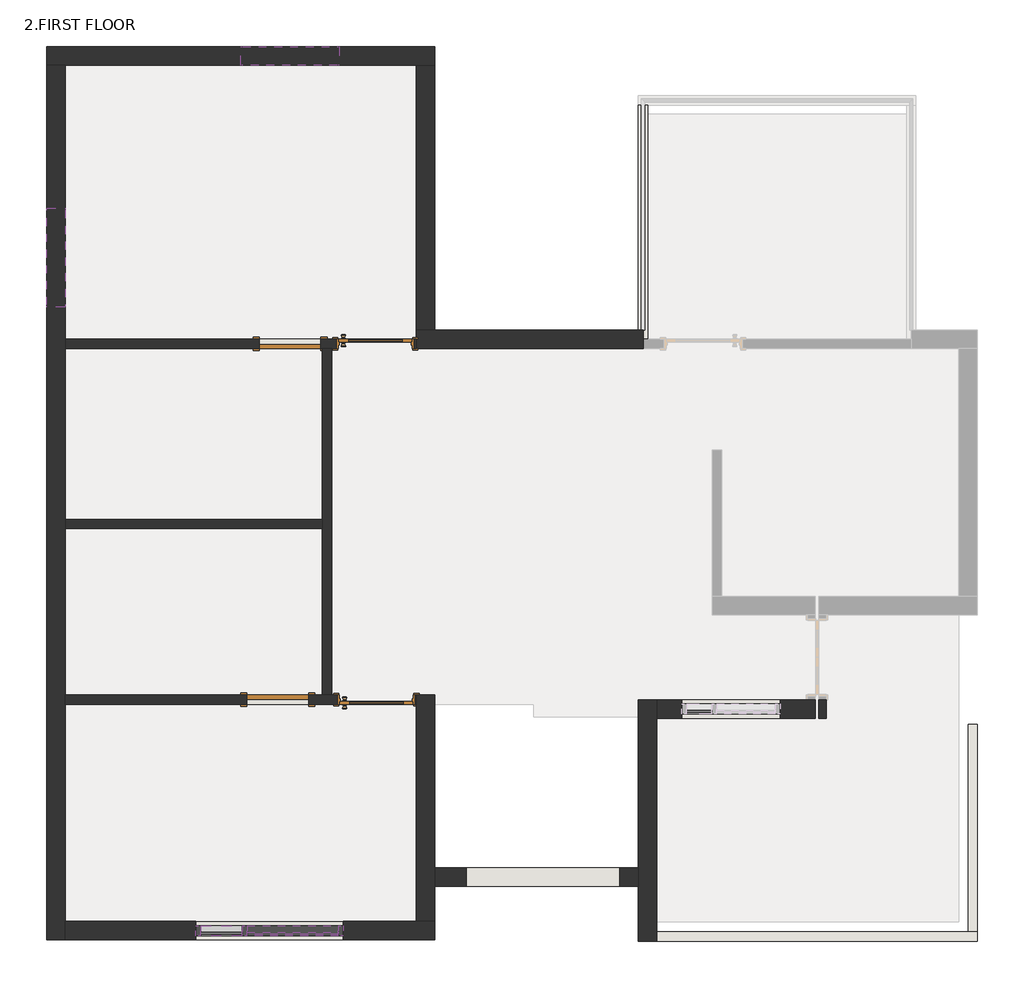
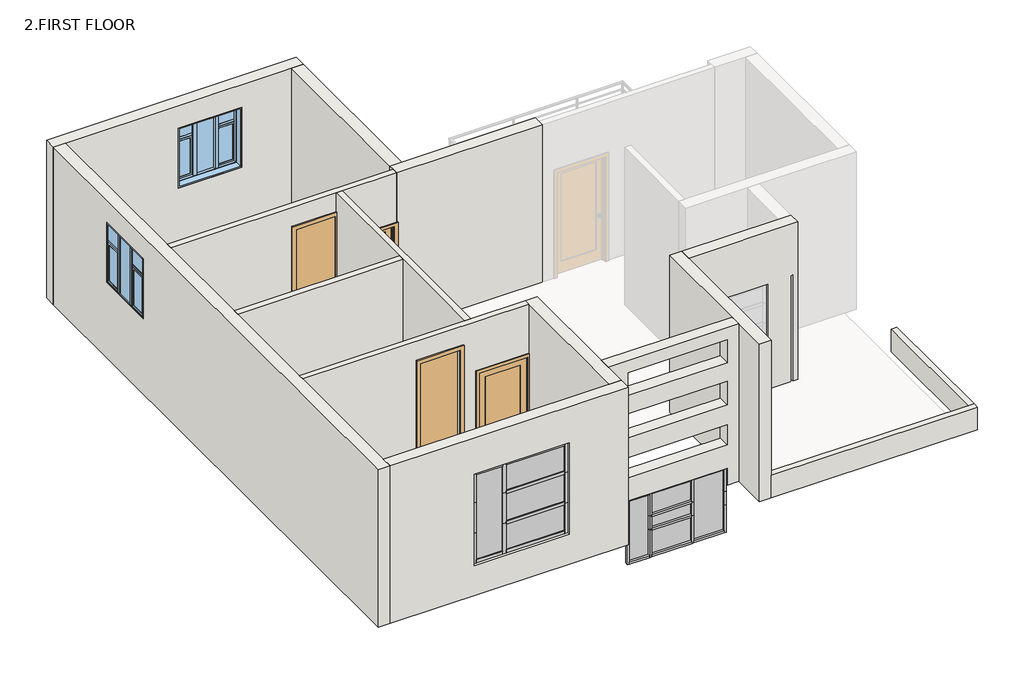
# One storey, part 1 of 2: 35 members, 16 walls, 10 plates, 4 doors, 2 windows.
"""IFC4 building model written with IfcOpenShell, lengths in millimetres."""

from ifc_helpers import new_model, si_unit, frame, origin, place, context, project, spatial, polyline, outline, extrude, faceted_brep, transform, mapped, element, save
from components import door_interior_single_1_panel_wood_4_x7_a3feeac7, door_interior_single_1_panel_wood_4_x7_3c6ab76a, door_214872d5, door_78caadf7, member_ade56e03, member_acd33549, member_5e1cd3ea, member_0748a5fc, member_494741c6, member_55e892ad, member_6a2c51b8, member_01c630bb, member_9157fb7c, member_e8de63ac, member_0b7646a3, member_e6b9f524, member_2cd1b1d9, member_866a01fa, member_c3a59c23, system_panel_glazed_06acdacc, system_panel_glazed_f6e37d5f, system_panel_glazed_d1e8daba, system_panel_glazed_58042333, system_panel_glazed_55b634e8, system_panel_glazed_1f22f3a7, system_panel_glazed_63219d49, system_panel_glazed_1b2af392, system_panel_glazed_fe088b68, window_casement_triple_side_transom_4_x4_fd24aed3

model = new_model("IFC4")

# Units and contexts
model_context = context("Model", 3, world=origin())
ifc_project = project(units=[si_unit("LENGTHUNIT", "METRE", prefix="MILLI")], contexts=[model_context])

# Site, building, storey
site = spatial("IfcSite", under=ifc_project)
building = spatial("IfcBuilding", under=site)
storey = spatial("IfcBuildingStorey", under=building, Name="2.FIRST FLOOR", Elevation=3810.0)

# Doors
placement = place(None, origin())
door_interior_single_1_panel_wood_4_x7_shape = door_interior_single_1_panel_wood_4_x7_a3feeac7(model_context)
element("IfcDoor", 1, ObjectType="Door-Interior-Single-1_Panel-Wood : 4'X7'", at=placement, inside=storey, context=model_context, shape_type="MappedRepresentation", body=[
    mapped(door_interior_single_1_panel_wood_4_x7_shape, transform((-3488.3749552, 2247.2410289, 3810.0), x_axis=(1.0, 0.0, 0.0), y_axis=(0.0, 1.0, 0.0), z_axis=(0.0, 0.0, 1.0))),
])
door_interior_single_1_panel_wood_4_x7_2_shape = door_interior_single_1_panel_wood_4_x7_3c6ab76a(model_context)
element("IfcDoor", 2, ObjectType="Door-Interior-Single-1_Panel-Wood : 4'X7'", at=placement, inside=storey, context=model_context, shape_type="MappedRepresentation", body=[
    mapped(door_interior_single_1_panel_wood_4_x7_2_shape, transform((-3501.0749552, 6654.1410289, 3810.0), x_axis=(1.0, 0.0, 0.0), y_axis=(0.0, 1.0, 0.0), z_axis=(0.0, 0.0, 1.0))),
])
door_shape = door_214872d5(model_context)
element("IfcDoor", 3, ObjectType="Single-Flush : 2'6\" X 7'", at=placement, inside=storey, context=model_context, shape_type="MappedRepresentation", body=[
    mapped(door_shape, transform((-4707.5749552, 2250.4160289, 4419.6), x_axis=(1.0, 0.0, 0.0), y_axis=(0.0, 1.0, 0.0), z_axis=(0.0, 0.0, 1.0))),
])
door_2_shape = door_78caadf7(model_context)
element("IfcDoor", 4, ObjectType="Single-Flush : 2'6\" X 7'", at=placement, inside=storey, context=model_context, shape_type="MappedRepresentation", body=[
    mapped(door_2_shape, transform((-4555.1749552, 6650.9660289, 4419.6), x_axis=(1.0, 0.0, 0.0), y_axis=(0.0, 1.0, 0.0), z_axis=(0.0, 0.0, 1.0))),
])

# Members
member_shape = member_ade56e03(model_context)
element("IfcMember", 5, ObjectType="Rectangular Mullion : 1.5\" x 2.5\" rectangular", at=placement, inside=storey, context=model_context, shape_type="MappedRepresentation", body=[
    mapped(member_shape, transform((-2380.0564961, 2.5160289, 4161.1588836), x_axis=(-1.0, 0.0, 0.0), y_axis=(0.0, -1.0, 0.0), z_axis=(0.0, 0.0, 1.0))),
])
element("IfcMember", 6, ObjectType="Rectangular Mullion : 1.5\" x 2.5\" rectangular", at=placement, inside=storey, context=model_context, shape_type="MappedRepresentation", body=[
    mapped(member_shape, transform((-478.4749552, 2.5160289, 3680.9734267), x_axis=(1.0, 0.0, 0.0), y_axis=(0.0, -1.0, 0.0), z_axis=(0.0, 0.0, -1.0))),
])
member_2_shape = member_acd33549(model_context)
element("IfcMember", 7, ObjectType="Rectangular Mullion : 1.5\" x 2.5\" rectangular", at=placement, inside=storey, context=model_context, shape_type="MappedRepresentation", body=[
    mapped(member_2_shape, transform((-478.4749552, 2.5160289, 2845.1879698), x_axis=(1.0, 0.0, 0.0), y_axis=(0.0, -1.0, 0.0), z_axis=(0.0, 0.0, -1.0))),
])
member_3_shape = member_5e1cd3ea(model_context)
element("IfcMember", 8, ObjectType="Rectangular Mullion : 1.5\" x 2.5\" rectangular", at=placement, inside=storey, context=model_context, shape_type="MappedRepresentation", body=[
    mapped(member_3_shape, transform((-2380.0564961, 2.5160289, 3680.9734267), x_axis=(-1.0, 0.0, 0.0), y_axis=(0.0, -1.0, 0.0), z_axis=(0.0, 0.0, 1.0))),
])
element("IfcMember", 9, ObjectType="Rectangular Mullion : 1.5\" x 2.5\" rectangular", at=placement, inside=storey, context=model_context, shape_type="MappedRepresentation", body=[
    mapped(member_3_shape, transform((-478.4749552, 2.5160289, 3402.3782744), x_axis=(1.0, 0.0, 0.0), y_axis=(0.0, -1.0, 0.0), z_axis=(0.0, 0.0, -1.0))),
])
element("IfcMember", 10, ObjectType="Rectangular Mullion : 1.5\" x 2.5\" rectangular", at=placement, inside=storey, context=model_context, shape_type="MappedRepresentation", body=[
    mapped(member_2_shape, transform((-2380.0564961, 2.5160289, 3402.3782744), x_axis=(-1.0, 0.0, 0.0), y_axis=(0.0, -1.0, 0.0), z_axis=(0.0, 0.0, 1.0))),
])
member_4_shape = member_0748a5fc(model_context)
element("IfcMember", 11, ObjectType="Rectangular Mullion : 1.5\" x 2.5\" rectangular", at=placement, inside=storey, context=model_context, shape_type="MappedRepresentation", body=[
    mapped(member_4_shape, transform((-1913.5749552, 2.5160289, 2845.1879698), x_axis=(0.0, 0.0, -1.0), y_axis=(0.0, -1.0, 0.0), z_axis=(-1.0, 0.0, 0.0))),
])
element("IfcMember", 12, ObjectType="Rectangular Mullion : 1.5\" x 2.5\" rectangular", at=placement, inside=storey, context=model_context, shape_type="MappedRepresentation", body=[
    mapped(member_4_shape, transform((-1138.8749552, 2.5160289, 4161.1588836), x_axis=(0.0, 0.0, 1.0), y_axis=(0.0, -1.0, 0.0), z_axis=(1.0, 0.0, 0.0))),
])
member_5_shape = member_494741c6(model_context)
element("IfcMember", 13, ObjectType="Rectangular Mullion : 1.5\" x 2.5\" rectangular", at=placement, inside=storey, context=model_context, shape_type="MappedRepresentation", body=[
    mapped(member_5_shape, transform((-1932.6249552, 2.5160289, 2845.1879698), x_axis=(1.0, 0.0, 0.0), y_axis=(0.0, -1.0, 0.0), z_axis=(0.0, 0.0, -1.0))),
])
element("IfcMember", 14, ObjectType="Rectangular Mullion : 1.5\" x 2.5\" rectangular", at=placement, inside=storey, context=model_context, shape_type="MappedRepresentation", body=[
    mapped(member_5_shape, transform((-1119.8249552, 2.5160289, 2845.1879698), x_axis=(1.0, 0.0, 0.0), y_axis=(0.0, -1.0, 0.0), z_axis=(0.0, 0.0, -1.0))),
])
member_6_shape = member_55e892ad(model_context)
element("IfcMember", 15, ObjectType="Rectangular Mullion : 1.5\" x 2.5\" rectangular", at=placement, inside=storey, context=model_context, shape_type="MappedRepresentation", body=[
    mapped(member_6_shape, transform((-1138.8749552, 2.5160289, 3680.9734267), x_axis=(0.0, 0.0, 1.0), y_axis=(0.0, -1.0, 0.0), z_axis=(1.0, 0.0, 0.0))),
])
element("IfcMember", 16, ObjectType="Rectangular Mullion : 1.5\" x 2.5\" rectangular", at=placement, inside=storey, context=model_context, shape_type="MappedRepresentation", body=[
    mapped(member_6_shape, transform((-1138.8749552, 2.5160289, 3402.3782744), x_axis=(0.0, 0.0, 1.0), y_axis=(0.0, -1.0, 0.0), z_axis=(1.0, 0.0, 0.0))),
])
member_7_shape = member_6a2c51b8(model_context)
element("IfcMember", 17, ObjectType="Rectangular Mullion : 1.5\" x 2.5\" rectangular", at=placement, inside=storey, context=model_context, shape_type="MappedRepresentation", body=[
    mapped(member_7_shape, transform((-1932.6249552, 2.5160289, 3680.9734267), x_axis=(1.0, 0.0, 0.0), y_axis=(0.0, -1.0, 0.0), z_axis=(0.0, 0.0, -1.0))),
])
element("IfcMember", 18, ObjectType="Rectangular Mullion : 1.5\" x 2.5\" rectangular", at=placement, inside=storey, context=model_context, shape_type="MappedRepresentation", body=[
    mapped(member_7_shape, transform((-1119.8249552, 2.5160289, 3680.9734267), x_axis=(1.0, 0.0, 0.0), y_axis=(0.0, -1.0, 0.0), z_axis=(0.0, 0.0, -1.0))),
])
member_8_shape = member_01c630bb(model_context)
element("IfcMember", 19, ObjectType="Rectangular Mullion : 1.5\" x 2.5\" rectangular", at=placement, inside=storey, context=model_context, shape_type="MappedRepresentation", body=[
    mapped(member_8_shape, transform((-1932.6249552, 2.5160289, 3402.3782744), x_axis=(1.0, 0.0, 0.0), y_axis=(0.0, -1.0, 0.0), z_axis=(0.0, 0.0, -1.0))),
])
element("IfcMember", 20, ObjectType="Rectangular Mullion : 1.5\" x 2.5\" rectangular", at=placement, inside=storey, context=model_context, shape_type="MappedRepresentation", body=[
    mapped(member_8_shape, transform((-1119.8249552, 2.5160289, 3402.3782744), x_axis=(1.0, 0.0, 0.0), y_axis=(0.0, -1.0, 0.0), z_axis=(0.0, 0.0, -1.0))),
])
member_9_shape = member_9157fb7c(model_context)
element("IfcMember", 21, ObjectType="Rectangular Mullion : 1.5\" x 2.5\" rectangular", at=placement, inside=storey, context=model_context, shape_type="MappedRepresentation", body=[
    mapped(member_9_shape, transform((-2341.9564961, 2.5160289, 2845.1879698), x_axis=(0.0, 0.0, -1.0), y_axis=(0.0, -1.0, 0.0), z_axis=(-1.0, 0.0, 0.0))),
])
element("IfcMember", 22, ObjectType="Rectangular Mullion : 1.5\" x 2.5\" rectangular", at=placement, inside=storey, context=model_context, shape_type="MappedRepresentation", body=[
    mapped(member_9_shape, transform((-1951.6749552, 2.5160289, 4161.1588836), x_axis=(0.0, 0.0, 1.0), y_axis=(0.0, -1.0, 0.0), z_axis=(1.0, 0.0, 0.0))),
])
member_10_shape = member_e8de63ac(model_context)
element("IfcMember", 23, ObjectType="Rectangular Mullion : 1.5\" x 2.5\" rectangular", at=placement, inside=storey, context=model_context, shape_type="MappedRepresentation", body=[
    mapped(member_10_shape, transform((-516.5749552, 2.5160289, 4161.1588836), x_axis=(0.0, 0.0, 1.0), y_axis=(0.0, -1.0, 0.0), z_axis=(1.0, 0.0, 0.0))),
])
element("IfcMember", 24, ObjectType="Rectangular Mullion : 1.5\" x 2.5\" rectangular", at=placement, inside=storey, context=model_context, shape_type="MappedRepresentation", body=[
    mapped(member_10_shape, transform((-1100.7749552, 2.5160289, 2845.1879698), x_axis=(0.0, 0.0, -1.0), y_axis=(0.0, -1.0, 0.0), z_axis=(-1.0, 0.0, 0.0))),
])
member_11_shape = member_0b7646a3(model_context)
element("IfcMember", 25, ObjectType="Rectangular Mullion : 2.5\" x 5\" rectangular", at=placement, inside=storey, context=model_context, shape_type="MappedRepresentation", body=[
    mapped(member_11_shape, transform((-5660.0749552, -607.0839711, 6273.8), x_axis=(0.0, 0.0, 1.0), y_axis=(0.0, 1.0, 0.0), z_axis=(-1.0, 0.0, 0.0))),
])
member_12_shape = member_e6b9f524(model_context)
element("IfcMember", 26, ObjectType="Rectangular Mullion : 2.5\" x 5\" rectangular", at=placement, inside=storey, context=model_context, shape_type="MappedRepresentation", body=[
    mapped(member_12_shape, transform((-3958.2749552, -607.0839711, 4419.6), x_axis=(0.0, 0.0, -1.0), y_axis=(0.0, 1.0, 0.0), z_axis=(1.0, 0.0, 0.0))),
])
member_13_shape = member_2cd1b1d9(model_context)
element("IfcMember", 27, ObjectType="Rectangular Mullion : 2.5\" x 5\" rectangular", at=placement, inside=storey, context=model_context, shape_type="MappedRepresentation", body=[
    mapped(member_13_shape, transform((-5113.9749552, -607.0839711, 4419.6), x_axis=(-1.0, 0.0, 0.0), y_axis=(0.0, 1.0, 0.0), z_axis=(0.0, 0.0, -1.0))),
])
member_14_shape = member_866a01fa(model_context)
element("IfcMember", 28, ObjectType="Rectangular Mullion : 2.5\" x 5\" rectangular", at=placement, inside=storey, context=model_context, shape_type="MappedRepresentation", body=[
    mapped(member_14_shape, transform((-5082.2249552, -607.0839711, 5655.7333333), x_axis=(0.0, 0.0, 1.0), y_axis=(0.0, 1.0, 0.0), z_axis=(-1.0, 0.0, 0.0))),
])
element("IfcMember", 29, ObjectType="Rectangular Mullion : 2.5\" x 5\" rectangular", at=placement, inside=storey, context=model_context, shape_type="MappedRepresentation", body=[
    mapped(member_14_shape, transform((-5082.2249552, -607.0839711, 5037.6666667), x_axis=(0.0, 0.0, 1.0), y_axis=(0.0, 1.0, 0.0), z_axis=(-1.0, 0.0, 0.0))),
])
element("IfcMember", 30, ObjectType="Rectangular Mullion : 2.5\" x 5\" rectangular", at=placement, inside=storey, context=model_context, shape_type="MappedRepresentation", body=[
    mapped(member_11_shape, transform((-5145.7249552, -607.0839711, 4419.6), x_axis=(0.0, 0.0, -1.0), y_axis=(0.0, 1.0, 0.0), z_axis=(1.0, 0.0, 0.0))),
])
element("IfcMember", 31, ObjectType="Rectangular Mullion : 2.5\" x 5\" rectangular", at=placement, inside=storey, context=model_context, shape_type="MappedRepresentation", body=[
    mapped(member_12_shape, transform((-5082.2249552, -607.0839711, 6273.8), x_axis=(0.0, 0.0, 1.0), y_axis=(0.0, 1.0, 0.0), z_axis=(-1.0, 0.0, 0.0))),
])
element("IfcMember", 32, ObjectType="Rectangular Mullion : 2.5\" x 5\" rectangular", at=placement, inside=storey, context=model_context, shape_type="MappedRepresentation", body=[
    mapped(member_13_shape, transform((-5113.9749552, -607.0839711, 5655.7333333), x_axis=(-1.0, 0.0, 0.0), y_axis=(0.0, 1.0, 0.0), z_axis=(0.0, 0.0, -1.0))),
])
element("IfcMember", 33, ObjectType="Rectangular Mullion : 2.5\" x 5\" rectangular", at=placement, inside=storey, context=model_context, shape_type="MappedRepresentation", body=[
    mapped(member_13_shape, transform((-5113.9749552, -607.0839711, 5037.6666667), x_axis=(-1.0, 0.0, 0.0), y_axis=(0.0, 1.0, 0.0), z_axis=(0.0, 0.0, -1.0))),
])
member_15_shape = member_c3a59c23(model_context)
element("IfcMember", 34, ObjectType="Rectangular Mullion : 2.5\" x 5\" rectangular", at=placement, inside=storey, context=model_context, shape_type="MappedRepresentation", body=[
    mapped(member_15_shape, transform((-3894.7749552, -607.0839711, 6273.8), x_axis=(1.0, 0.0, 0.0), y_axis=(0.0, 1.0, 0.0), z_axis=(0.0, 0.0, 1.0))),
])
element("IfcMember", 35, ObjectType="Rectangular Mullion : 2.5\" x 5\" rectangular", at=placement, inside=storey, context=model_context, shape_type="MappedRepresentation", body=[
    mapped(member_15_shape, transform((-5723.5749552, -607.0839711, 4419.6), x_axis=(-1.0, 0.0, 0.0), y_axis=(0.0, 1.0, 0.0), z_axis=(0.0, 0.0, -1.0))),
])
element("IfcMember", 36, ObjectType="Rectangular Mullion : 2.5\" x 5\" rectangular", at=placement, inside=storey, context=model_context, shape_type="MappedRepresentation", body=[
    mapped(member_15_shape, transform((-5723.5749552, -607.0839711, 5655.7333333), x_axis=(-1.0, 0.0, 0.0), y_axis=(0.0, 1.0, 0.0), z_axis=(0.0, 0.0, -1.0))),
])
element("IfcMember", 37, ObjectType="Rectangular Mullion : 2.5\" x 5\" rectangular", at=placement, inside=storey, context=model_context, shape_type="MappedRepresentation", body=[
    mapped(member_15_shape, transform((-5723.5749552, -607.0839711, 5037.6666667), x_axis=(-1.0, 0.0, 0.0), y_axis=(0.0, 1.0, 0.0), z_axis=(0.0, 0.0, -1.0))),
])
element("IfcMember", 38, ObjectType="Rectangular Mullion : 2.5\" x 5\" rectangular", at=placement, inside=storey, context=model_context, shape_type="MappedRepresentation", body=[
    mapped(member_15_shape, transform((-3894.7749552, -607.0839711, 5655.7333333), x_axis=(1.0, 0.0, 0.0), y_axis=(0.0, 1.0, 0.0), z_axis=(0.0, 0.0, 1.0))),
])
element("IfcMember", 39, ObjectType="Rectangular Mullion : 2.5\" x 5\" rectangular", at=placement, inside=storey, context=model_context, shape_type="MappedRepresentation", body=[
    mapped(member_15_shape, transform((-3894.7749552, -607.0839711, 5037.6666667), x_axis=(1.0, 0.0, 0.0), y_axis=(0.0, 1.0, 0.0), z_axis=(0.0, 0.0, 1.0))),
])

# Plates
system_panel_glazed_shape = system_panel_glazed_06acdacc(model_context)
element("IfcPlate", 40, ObjectType="System Panel : Glazed", at=placement, inside=storey, context=model_context, shape_type="MappedRepresentation", body=[
    mapped(system_panel_glazed_shape, transform((-4520.2499552, -607.0839711, 4483.1), x_axis=(-1.0, 0.0, 0.0), y_axis=(0.0, -1.0, 0.0), z_axis=(0.0, 0.0, 1.0))),
])
element("IfcPlate", 41, ObjectType="System Panel : Glazed", at=placement, inside=storey, context=model_context, shape_type="MappedRepresentation", body=[
    mapped(system_panel_glazed_shape, transform((-4520.2499552, -607.0839711, 5687.4833333), x_axis=(-1.0, 0.0, 0.0), y_axis=(0.0, -1.0, 0.0), z_axis=(0.0, 0.0, 1.0))),
])
system_panel_glazed_2_shape = system_panel_glazed_f6e37d5f(model_context)
element("IfcPlate", 42, ObjectType="System Panel : Glazed", at=placement, inside=storey, context=model_context, shape_type="MappedRepresentation", body=[
    mapped(system_panel_glazed_2_shape, transform((-5402.8999552, -607.0839711, 4483.1), x_axis=(-1.0, 0.0, 0.0), y_axis=(0.0, -1.0, 0.0), z_axis=(0.0, 0.0, 1.0))),
])
system_panel_glazed_3_shape = system_panel_glazed_d1e8daba(model_context)
element("IfcPlate", 43, ObjectType="System Panel : Glazed", at=placement, inside=storey, context=model_context, shape_type="MappedRepresentation", body=[
    mapped(system_panel_glazed_3_shape, transform((-4520.2499552, -607.0839711, 5069.4166667), x_axis=(-1.0, 0.0, 0.0), y_axis=(0.0, -1.0, 0.0), z_axis=(0.0, 0.0, 1.0))),
])
system_panel_glazed_4_shape = system_panel_glazed_58042333(model_context)
element("IfcPlate", 44, ObjectType="System Panel : Glazed", at=placement, inside=storey, context=model_context, shape_type="MappedRepresentation", body=[
    mapped(system_panel_glazed_4_shape, transform((502.6000448, 2136.1160289, 4787.9), x_axis=(-1.0, 0.0, 0.0), y_axis=(0.0, -1.0, 0.0), z_axis=(0.0, 0.0, 1.0))),
])
system_panel_glazed_5_shape = system_panel_glazed_55b634e8(model_context)
element("IfcPlate", 45, ObjectType="System Panel : Glazed", at=placement, inside=storey, context=model_context, shape_type="MappedRepresentation", body=[
    mapped(system_panel_glazed_5_shape, transform((-1526.2249552, 2.5160289, 2883.2879698), x_axis=(1.0, 0.0, 0.0), y_axis=(0.0, 1.0, 0.0), z_axis=(0.0, 0.0, 1.0))),
])
system_panel_glazed_6_shape = system_panel_glazed_1f22f3a7(model_context)
element("IfcPlate", 46, ObjectType="System Panel : Glazed", at=placement, inside=storey, context=model_context, shape_type="MappedRepresentation", body=[
    mapped(system_panel_glazed_6_shape, transform((-1526.2249552, 2.5160289, 3700.0234267), x_axis=(1.0, 0.0, 0.0), y_axis=(0.0, 1.0, 0.0), z_axis=(0.0, 0.0, 1.0))),
])
system_panel_glazed_7_shape = system_panel_glazed_63219d49(model_context)
element("IfcPlate", 47, ObjectType="System Panel : Glazed", at=placement, inside=storey, context=model_context, shape_type="MappedRepresentation", body=[
    mapped(system_panel_glazed_7_shape, transform((-1526.2249552, 2.5160289, 3421.4282744), x_axis=(1.0, 0.0, 0.0), y_axis=(0.0, 1.0, 0.0), z_axis=(0.0, 0.0, 1.0))),
])
system_panel_glazed_8_shape = system_panel_glazed_1b2af392(model_context)
element("IfcPlate", 48, ObjectType="System Panel : Glazed", at=placement, inside=storey, context=model_context, shape_type="MappedRepresentation", body=[
    mapped(system_panel_glazed_8_shape, transform((-2146.8157257, 2.5160289, 2883.2879698), x_axis=(1.0, 0.0, 0.0), y_axis=(0.0, 1.0, 0.0), z_axis=(0.0, 0.0, 1.0))),
])
system_panel_glazed_9_shape = system_panel_glazed_fe088b68(model_context)
element("IfcPlate", 49, ObjectType="System Panel : Glazed", at=placement, inside=storey, context=model_context, shape_type="MappedRepresentation", body=[
    mapped(system_panel_glazed_9_shape, transform((-808.6749552, 2.5160289, 2883.2879698), x_axis=(1.0, 0.0, 0.0), y_axis=(0.0, 1.0, 0.0), z_axis=(0.0, 0.0, 1.0))),
])

# Walls
element("IfcWall", 50, ObjectType="4.5\" wall", at=placement, inside=storey, context=model_context, shape_type="Brep", body=[
    faceted_brep([(-7336.4749552, 6708.1160289, 7010.4), (-2993.0749552, 6708.1160289, 7010.4), (-2993.0749552, 6708.1160289, 3810.0), (-3018.4749552, 6708.1160289, 3810.0), (-3018.4749552, 6708.1160289, 5969.0), (-3983.6749552, 6708.1160289, 5969.0), (-3983.6749552, 6708.1160289, 3810.0), (-7336.4749552, 6708.1160289, 3810.0), (-4936.1749552, 6708.1160289, 4419.6), (-4174.1749552, 6708.1160289, 4419.6), (-4174.1749552, 6708.1160289, 6553.2), (-4936.1749552, 6708.1160289, 6553.2), (-2993.0749552, 6593.8160289, 7010.4), (-4040.8249552, 6593.8160289, 7010.4), (-4155.1249552, 6593.8160289, 7010.4), (-7336.4749552, 6593.8160289, 7010.4), (-7336.4749552, 6593.8160289, 3810.0), (-4155.1249552, 6593.8160289, 3810.0), (-4040.8249552, 6593.8160289, 3810.0), (-3983.6749552, 6593.8160289, 3810.0), (-3983.6749552, 6593.8160289, 5969.0), (-3018.4749552, 6593.8160289, 5969.0), (-3018.4749552, 6593.8160289, 3810.0), (-2993.0749552, 6593.8160289, 3810.0), (-4174.1749552, 6593.8160289, 4419.6), (-4936.1749552, 6593.8160289, 4419.6), (-4936.1749552, 6593.8160289, 6553.2), (-4174.1749552, 6593.8160289, 6553.2)], [[[0, 1, 2, 3, 4, 5, 6, 7], [8, 9, 10, 11]], [[12, 13, 14, 15, 16, 17, 18, 19, 20, 21, 22, 23], [24, 25, 26, 27]], [[2, 23, 22, 3]], [[16, 7, 6, 19, 18, 17]], [[1, 0, 15, 14, 13, 12]], [[21, 4, 3, 22]], [[4, 21, 20, 5]], [[5, 20, 19, 6]], [[9, 8, 25, 24]], [[10, 9, 24, 27]], [[11, 10, 27, 26]], [[8, 11, 26, 25]], [[2, 1, 12, 23]], [[0, 7, 16, 15]]]),
])
element("IfcWall", 51, ObjectType="4.5\" wall", at=placement, inside=storey, context=model_context, shape_type="Brep", body=[
    faceted_brep([(-4155.1249552, 6593.8160289, 3810.0), (-4155.1249552, 4479.2660289, 3810.0), (-4155.1249552, 4364.9660289, 3810.0), (-4155.1249552, 2307.5660289, 3810.0), (-4155.1249552, 2307.5660289, 7010.4), (-4155.1249552, 4364.9660289, 7010.4), (-4155.1249552, 4479.2660289, 7010.4), (-4155.1249552, 6593.8160289, 7010.4), (-4040.8249552, 6593.8160289, 3810.0), (-4040.8249552, 6593.8160289, 7010.4), (-4040.8249552, 2307.5660289, 7010.4), (-4040.8249552, 2307.5660289, 3810.0)], [[[0, 1, 2, 3, 4, 5, 6, 7]], [[8, 9, 10, 11]], [[3, 2, 1, 0, 8, 11]], [[7, 6, 5, 4, 10, 9]], [[0, 7, 9, 8]], [[4, 3, 11, 10]]]),
])
element("IfcWall", 52, ObjectType="4.5\" wall", at=placement, inside=storey, context=model_context, shape_type="Brep", body=[
    faceted_brep([(-7336.4749552, 2307.5660289, 7010.4), (-4155.1249552, 2307.5660289, 7010.4), (-4040.8249552, 2307.5660289, 7010.4), (-2993.0749552, 2307.5660289, 7010.4), (-2993.0749552, 2307.5660289, 3810.0), (-3005.7749552, 2307.5660289, 3810.0), (-3005.7749552, 2307.5660289, 5969.0), (-3970.9749552, 2307.5660289, 5969.0), (-3970.9749552, 2307.5660289, 3810.0), (-4040.8249552, 2307.5660289, 3810.0), (-4155.1249552, 2307.5660289, 3810.0), (-7336.4749552, 2307.5660289, 3810.0), (-5088.5749552, 2307.5660289, 4419.6), (-4326.5749552, 2307.5660289, 4419.6), (-4326.5749552, 2307.5660289, 6553.2), (-5088.5749552, 2307.5660289, 6553.2), (-2993.0749552, 2193.2660289, 7010.4), (-7336.4749552, 2193.2660289, 7010.4), (-7336.4749552, 2193.2660289, 3810.0), (-3970.9749552, 2193.2660289, 3810.0), (-3970.9749552, 2193.2660289, 5969.0), (-3005.7749552, 2193.2660289, 5969.0), (-3005.7749552, 2193.2660289, 3810.0), (-2993.0749552, 2193.2660289, 3810.0), (-4326.5749552, 2193.2660289, 4419.6), (-5088.5749552, 2193.2660289, 4419.6), (-5088.5749552, 2193.2660289, 6553.2), (-4326.5749552, 2193.2660289, 6553.2)], [[[0, 1, 2, 3, 4, 5, 6, 7, 8, 9, 10, 11], [12, 13, 14, 15]], [[16, 17, 18, 19, 20, 21, 22, 23], [24, 25, 26, 27]], [[4, 23, 22, 5]], [[18, 11, 10, 9, 8, 19]], [[3, 2, 1, 0, 17, 16]], [[21, 6, 5, 22]], [[6, 21, 20, 7]], [[7, 20, 19, 8]], [[13, 12, 25, 24]], [[14, 13, 24, 27]], [[15, 14, 27, 26]], [[12, 15, 26, 25]], [[4, 3, 16, 23]], [[0, 11, 18, 17]]]),
])
element("IfcWall", 53, ObjectType="4.5\" wall", at=placement, inside=storey, context=model_context, shape_type="SweptSolid", body=[
    extrude(outline(polyline([(-7336.4749552, 4479.2660289), (-4155.1249552, 4479.2660289), (-4155.1249552, 4364.9660289), (-7336.4749552, 4364.9660289), (-7336.4749552, 4479.2660289)])), frame((0.0, 0.0, 3810.0), z_axis=(0.0, 0.0, 1.0), x_axis=(1.0, 0.0, 0.0)), (0.0, 0.0, 1.0), 3200.4),
])
element("IfcWall", 54, ObjectType="4.5\" wall", at=placement, inside=storey, context=model_context, shape_type="Brep", body=[
    faceted_brep([(-21.2749552, -734.0839711, 3810.0), (3941.1250448, -734.0839711, 3810.0), (3941.1250448, -734.0839711, 4267.2), (-21.2749552, -734.0839711, 4267.2), (-21.2749552, -619.7839711, 3810.0), (-21.2749552, -619.7839711, 4267.2), (3826.8250448, -619.7839711, 4267.2), (3941.1250448, -619.7839711, 4267.2), (3941.1250448, -619.7839711, 3810.0), (3826.8250448, -619.7839711, 3810.0)], [[[0, 1, 2, 3]], [[4, 5, 6, 7, 8, 9]], [[1, 0, 4, 9, 8]], [[3, 2, 7, 6, 5]], [[0, 3, 5, 4]], [[2, 1, 8, 7]]]),
])
element("IfcWall", 55, ObjectType="4.5\" wall", at=placement, inside=storey, context=model_context, shape_type="SweptSolid", body=[
    extrude(outline(polyline([(3941.1250448, 1945.6160289), (3941.1250448, -619.7839711), (3826.8250448, -619.7839711), (3826.8250448, 1945.6160289), (3941.1250448, 1945.6160289)])), frame((0.0, 0.0, 3810.0), z_axis=(0.0, 0.0, 1.0), x_axis=(1.0, 0.0, 0.0)), (0.0, 0.0, 1.0), 457.2),
])
element("IfcWall", 56, ObjectType="4.5\" wall", at=placement, inside=storey, context=model_context, shape_type="SweptSolid", body=[
    extrude(outline(polyline([(-249.8749552, 6822.4160289), (-249.8749552, 9603.7160289), (-135.5749552, 9603.7160289), (-135.5749552, 6708.1160289), (-192.7249552, 6708.1160289), (-192.7249552, 6822.4160289), (-249.8749552, 6822.4160289)])), frame((0.0, 0.0, 3810.0), z_axis=(0.0, 0.0, 1.0), x_axis=(1.0, 0.0, 0.0)), (0.0, 0.0, 1.0), 304.8),
])
element("IfcWall", 57, ObjectType="9\" wall", at=placement, inside=storey, context=model_context, shape_type="Brep", body=[
    faceted_brep([(-2764.4749552, 10327.6160289, 3810.0), (-7565.0749552, 10327.6160289, 3810.0), (-7565.0749552, 10327.6160289, 7010.4), (-2764.4749552, 10327.6160289, 7010.4), (-3945.5749552, 10327.6160289, 6553.2), (-5164.7749552, 10327.6160289, 6553.2), (-5164.7749552, 10327.6160289, 5334.0), (-3945.5749552, 10327.6160289, 5334.0), (-2764.4749552, 10099.0160289, 3810.0), (-2764.4749552, 10099.0160289, 7010.4), (-2993.0749552, 10099.0160289, 7010.4), (-7336.4749552, 10099.0160289, 7010.4), (-7565.0749552, 10099.0160289, 7010.4), (-7565.0749552, 10099.0160289, 3810.0), (-7336.4749552, 10099.0160289, 3810.0), (-2993.0749552, 10099.0160289, 3810.0), (-3945.5749552, 10099.0160289, 6553.2), (-3945.5749552, 10099.0160289, 5334.0), (-5164.7749552, 10099.0160289, 5334.0), (-5164.7749552, 10099.0160289, 6553.2)], [[[0, 1, 2, 3], [4, 5, 6, 7]], [[8, 9, 10, 11, 12, 13, 14, 15], [16, 17, 18, 19]], [[1, 0, 8, 15, 14, 13]], [[3, 2, 12, 11, 10, 9]], [[2, 1, 13, 12]], [[0, 3, 9, 8]], [[17, 16, 4, 7]], [[18, 17, 7, 6]], [[19, 18, 6, 5]], [[16, 19, 5, 4]]]),
])
element("IfcWall", 58, ObjectType="9\" wall", at=placement, inside=storey, context=model_context, shape_type="Brep", body=[
    faceted_brep([(-7565.0749552, 10099.0160289, 3810.0), (-7565.0749552, -721.3839711, 3810.0), (-7565.0749552, -721.3839711, 7010.4), (-7565.0749552, 10099.0160289, 7010.4), (-7565.0749552, 8327.3660289, 6553.2), (-7565.0749552, 7108.1660289, 6553.2), (-7565.0749552, 7108.1660289, 5334.0), (-7565.0749552, 8327.3660289, 5334.0), (-7336.4749552, 10099.0160289, 3810.0), (-7336.4749552, 10099.0160289, 7010.4), (-7336.4749552, 6708.1160289, 7010.4), (-7336.4749552, 6593.8160289, 7010.4), (-7336.4749552, 4479.2660289, 7010.4), (-7336.4749552, 4364.9660289, 7010.4), (-7336.4749552, 2307.5660289, 7010.4), (-7336.4749552, 2193.2660289, 7010.4), (-7336.4749552, -492.7839711, 7010.4), (-7336.4749552, -721.3839711, 7010.4), (-7336.4749552, -721.3839711, 3810.0), (-7336.4749552, -492.7839711, 3810.0), (-7336.4749552, 2193.2660289, 3810.0), (-7336.4749552, 2307.5660289, 3810.0), (-7336.4749552, 4364.9660289, 3810.0), (-7336.4749552, 4479.2660289, 3810.0), (-7336.4749552, 6593.8160289, 3810.0), (-7336.4749552, 6708.1160289, 3810.0), (-7336.4749552, 8327.3660289, 6553.2), (-7336.4749552, 8327.3660289, 5334.0), (-7336.4749552, 7108.1660289, 5334.0), (-7336.4749552, 7108.1660289, 6553.2)], [[[0, 1, 2, 3], [4, 5, 6, 7]], [[8, 9, 10, 11, 12, 13, 14, 15, 16, 17, 18, 19, 20, 21, 22, 23, 24, 25], [26, 27, 28, 29]], [[1, 0, 8, 25, 24, 23, 22, 21, 20, 19, 18]], [[3, 2, 17, 16, 15, 14, 13, 12, 11, 10, 9]], [[0, 3, 9, 8]], [[2, 1, 18, 17]], [[27, 26, 4, 7]], [[28, 27, 7, 6]], [[29, 28, 6, 5]], [[26, 29, 5, 4]]]),
])
element("IfcWall", 59, ObjectType="9\" wall", at=placement, inside=storey, context=model_context, shape_type="Brep", body=[
    faceted_brep([(-7336.4749552, -721.3839711, 3810.0), (-2764.4749552, -721.3839711, 3810.0), (-2764.4749552, -721.3839711, 7010.4), (-7336.4749552, -721.3839711, 7010.4), (-3894.7749552, -721.3839711, 6273.8), (-3894.7749552, -721.3839711, 4419.6), (-5723.5749552, -721.3839711, 4419.6), (-5723.5749552, -721.3839711, 6273.8), (-2764.4749552, -492.7839711, 3810.0), (-2993.0749552, -492.7839711, 3810.0), (-7336.4749552, -492.7839711, 3810.0), (-7336.4749552, -492.7839711, 7010.4), (-2993.0749552, -492.7839711, 7010.4), (-2764.4749552, -492.7839711, 7010.4), (-3894.7749552, -492.7839711, 4419.6), (-3894.7749552, -492.7839711, 6273.8), (-5723.5749552, -492.7839711, 6273.8), (-5723.5749552, -492.7839711, 4419.6)], [[[0, 1, 2, 3], [4, 5, 6, 7]], [[8, 9, 10, 11, 12, 13], [14, 15, 16, 17]], [[1, 0, 10, 9, 8]], [[3, 2, 13, 12, 11]], [[0, 3, 11, 10]], [[2, 1, 8, 13]], [[14, 5, 4, 15]], [[15, 4, 7, 16]], [[16, 7, 6, 17]], [[5, 14, 17, 6]]]),
])
element("IfcWall", 60, ObjectType="9\" wall", at=placement, inside=storey, context=model_context, shape_type="Brep", body=[
    faceted_brep([(-2764.4749552, -492.7839711, 3810.0), (-2764.4749552, -54.6339711, 3810.0), (-2764.4749552, 173.9660289, 3810.0), (-2764.4749552, 2307.5660289, 3810.0), (-2764.4749552, 2307.5660289, 7010.4), (-2764.4749552, 173.9660289, 7010.4), (-2764.4749552, -54.6339711, 7010.4), (-2764.4749552, -492.7839711, 7010.4), (-2993.0749552, -492.7839711, 3810.0), (-2993.0749552, -492.7839711, 7010.4), (-2993.0749552, 2193.2660289, 7010.4), (-2993.0749552, 2307.5660289, 7010.4), (-2993.0749552, 2307.5660289, 3810.0), (-2993.0749552, 2193.2660289, 3810.0)], [[[0, 1, 2, 3, 4, 5, 6, 7]], [[8, 9, 10, 11, 12, 13]], [[3, 2, 1, 0, 8, 13, 12]], [[7, 6, 5, 4, 11, 10, 9]], [[0, 7, 9, 8]], [[4, 3, 12, 11]]]),
])
element("IfcWall", 61, ObjectType="9\" wall", at=placement, inside=storey, context=model_context, shape_type="SweptSolid", body=[
    extrude(outline(polyline([(7010.4, -249.8749552), (7010.4, -2764.4749552), (3810.0, -2764.4749552), (3810.0, -2380.0564961), (4161.1588836, -2380.0564961), (4161.1588836, -478.4749552), (3810.0, -478.4749552), (3810.0, -249.8749552), (7010.4, -249.8749552)]), holes=[polyline([(6307.1112081, -2380.0564961), (6765.5847346, -2380.0564961), (6765.5847346, -478.4749552), (6307.1112081, -478.4749552), (6307.1112081, -2380.0564961)]), polyline([(5446.3786483, -2380.0564961), (5927.3906231, -2380.0564961), (5927.3906231, -478.4749552), (5446.3786483, -478.4749552), (5446.3786483, -2380.0564961)]), polyline([(4633.507951, -2380.0564961), (5039.9421734, -2380.0564961), (5039.9421734, -478.4749552), (4633.507951, -478.4749552), (4633.507951, -2380.0564961)])]), frame((0.0, -54.6339711, 0.0), z_axis=(0.0, 1.0, 0.0), x_axis=(0.0, 0.0, 1.0)), (0.0, 0.0, 1.0), 228.6),
])
element("IfcWall", 62, ObjectType="9\" wall", at=placement, inside=storey, context=model_context, shape_type="Brep", body=[
    faceted_brep([(-21.2749552, -734.0839711, 3810.0), (-21.2749552, -619.7839711, 3810.0), (-21.2749552, 2021.8160289, 3810.0), (-21.2749552, 2250.4160289, 3810.0), (-21.2749552, 2250.4160289, 7010.4), (-21.2749552, 2021.8160289, 7010.4), (-21.2749552, -734.0839711, 7010.4), (-21.2749552, -734.0839711, 4267.2), (-249.8749552, -734.0839711, 3810.0), (-249.8749552, -734.0839711, 7010.4), (-249.8749552, -54.6339711, 7010.4), (-249.8749552, 173.9660289, 7010.4), (-249.8749552, 2250.4160289, 7010.4), (-249.8749552, 2250.4160289, 3810.0), (-249.8749552, 173.9660289, 3810.0), (-249.8749552, -54.6339711, 3810.0)], [[[0, 1, 2, 3, 4, 5, 6, 7]], [[8, 9, 10, 11, 12, 13, 14, 15]], [[3, 2, 1, 0, 8, 15, 14, 13]], [[6, 5, 4, 12, 11, 10, 9]], [[4, 3, 13, 12]], [[0, 7, 6, 9, 8]]]),
])
element("IfcWall", 63, ObjectType="9\" wall", at=placement, inside=storey, context=model_context, shape_type="Brep", body=[
    faceted_brep([(-192.7249552, 6822.4160289, 7010.4), (-192.7249552, 6822.4160289, 6553.2), (-192.7249552, 6822.4160289, 4114.8), (-192.7249552, 6822.4160289, 3810.0), (-249.8749552, 6822.4160289, 3810.0), (-2764.4749552, 6822.4160289, 3810.0), (-2993.0749552, 6822.4160289, 3810.0), (-2993.0749552, 6822.4160289, 7010.4), (-2878.7749552, 6822.4160289, 7010.4), (-2764.4749552, 6822.4160289, 7010.4), (-192.7249552, 6593.8160289, 3810.0), (-192.7249552, 6593.8160289, 7010.4), (-2993.0749552, 6593.8160289, 7010.4), (-2993.0749552, 6593.8160289, 3810.0), (-192.7249552, 6708.1160289, 3810.0), (-2993.0749552, 6708.1160289, 3810.0), (-2993.0749552, 6708.1160289, 7010.4), (-192.7249552, 6708.1160289, 7010.4)], [[[0, 1, 2, 3, 4, 5, 6, 7, 8, 9]], [[10, 11, 12, 13]], [[6, 5, 4, 3, 14, 10, 13, 15]], [[0, 9, 8, 7, 16, 12, 11, 17]], [[7, 6, 15, 13, 12, 16]], [[0, 17, 11, 10, 14, 3, 2, 1]]]),
])
element("IfcWall", 64, ObjectType="9\" wall", at=placement, inside=storey, context=model_context, shape_type="SweptSolid", body=[
    extrude(outline(polyline([(-2764.4749552, 10099.0160289), (-2764.4749552, 6822.4160289), (-2993.0749552, 6822.4160289), (-2993.0749552, 10099.0160289), (-2764.4749552, 10099.0160289)])), frame((0.0, 0.0, 3810.0), z_axis=(0.0, 0.0, 1.0), x_axis=(1.0, 0.0, 0.0)), (0.0, 0.0, 1.0), 3200.4),
])
element("IfcWall", 65, ObjectType="9\" wall", at=placement, inside=storey, context=model_context, shape_type="Brep", body=[
    faceted_brep([(2074.2250448, 2021.8160289, 7010.4), (-21.2749552, 2021.8160289, 7010.4), (-21.2749552, 2021.8160289, 3810.0), (1939.2875448, 2021.8160289, 3810.0), (1939.2875448, 2021.8160289, 5969.0), (1980.5625448, 2021.8160289, 5969.0), (1980.5625448, 2021.8160289, 3810.0), (2074.2250448, 2021.8160289, 3810.0), (1502.7250448, 2021.8160289, 5943.6), (1502.7250448, 2021.8160289, 4724.4), (283.5250448, 2021.8160289, 4724.4), (283.5250448, 2021.8160289, 5943.6), (-21.2749552, 2250.4160289, 7010.4), (1845.6250448, 2250.4160289, 7010.4), (2074.2250448, 2250.4160289, 7010.4), (2074.2250448, 2250.4160289, 3810.0), (1980.5625448, 2250.4160289, 3810.0), (1980.5625448, 2250.4160289, 5969.0), (1939.2875448, 2250.4160289, 5969.0), (1939.2875448, 2250.4160289, 3810.0), (1845.6250448, 2250.4160289, 3810.0), (-21.2749552, 2250.4160289, 3810.0), (1502.7250448, 2250.4160289, 4724.4), (1502.7250448, 2250.4160289, 5943.6), (283.5250448, 2250.4160289, 5943.6), (283.5250448, 2250.4160289, 4724.4)], [[[0, 1, 2, 3, 4, 5, 6, 7], [8, 9, 10, 11]], [[12, 13, 14, 15, 16, 17, 18, 19, 20, 21], [22, 23, 24, 25]], [[2, 21, 20, 19, 3]], [[15, 7, 6, 16]], [[1, 0, 14, 13, 12]], [[2, 1, 12, 21]], [[0, 7, 15, 14]], [[4, 18, 17, 5]], [[5, 17, 16, 6]], [[18, 4, 3, 19]], [[22, 9, 8, 23]], [[23, 8, 11, 24]], [[24, 11, 10, 25]], [[9, 22, 25, 10]]]),
])

# Windows
window_casement_triple_side_transom_4_x4_shape = window_casement_triple_side_transom_4_x4_fd24aed3(model_context)
element("IfcWindow", 66, ObjectType="Window-Casement-Triple-Side-Transom : 4'x4'", at=placement, inside=storey, context=model_context, shape_type="MappedRepresentation", body=[
    mapped(window_casement_triple_side_transom_4_x4_shape, transform((-4555.1749552, 10213.3160289, 4419.6), x_axis=(1.0, 0.0, 0.0), y_axis=(0.0, 1.0, 0.0), z_axis=(0.0, 0.0, 1.0))),
])
element("IfcWindow", 67, ObjectType="Window-Casement-Triple-Side-Transom : 4'x4'", at=placement, inside=storey, context=model_context, shape_type="MappedRepresentation", body=[
    mapped(window_casement_triple_side_transom_4_x4_shape, transform((-7450.7749552, 7717.7660289, 4419.6), x_axis=(0.0, 1.0, 0.0), y_axis=(-1.0, 0.0, 0.0), z_axis=(0.0, 0.0, 1.0))),
])

save(model, "model.ifc")

# Revit data of these elements
# Type "Door-Interior-Single-1_Panel-Wood : 4'X7'"
#   Type Mark = "9"
#   Assembly Code = "C1020300"
#   Analytic Construction = "Wooden"
#   Top Rail = 0' - 4 11/16"
#   Thickness = 0' - 1 3/8"
#   Thermal Resistance (R) = 2.5876 (h·ft²·°F)/BTU
#   Swing Angle [instance default] = 90.00°
#   Stiles = 0' - 4 3/4"
#   Rough Width = 3' - 2"
#   Rough Height = 7' - 1"
#   Height = 7' - 0"
#   Width = 3' - 0"
#   Heat Transfer Coefficient (U) = 0.3865 BTU/(h·ft²·°F)
#   Bottom Rail = 0' - 9 1/8"
#   Trim Material = Cherry
#   Panel Material = Cherry
#   Frame Material = Cherry
#   Door Handle Material = Aluminum
#   Visual Light Transmittance = 0
#   Solar Heat Gain Coefficient = 0
#   Wall Closure = (empty or 0)
#   Function = (empty or 0)
# Type "Single-Flush : 2'6\" X 7'"
#   Type Mark = "14"
#   Construction Type Id = "MDOOR"
#   Assembly Code = "C1020"
#   Analytic Construction = "Metal"
#   Thickness = 0' - 2"
#   Heat Transfer Coefficient (U) = 0.651978 BTU/(h·ft²·°F)
#   Height = 7' - 0"
#   Trim Projection Ext = 0' - 1"
#   Trim Projection Int = 0' - 1"
#   Trim Width = 0' - 3"
#   Width = 2' - 6"
#   Define Thermal Properties by = 1
#   Door Material = Door - Panel
#   Frame Material = Door - Frame
#   Visual Light Transmittance = 0
#   Solar Heat Gain Coefficient = 0
#   Function = (empty or 0)
#   Wall Closure = (empty or 0)
# Type "Rectangular Mullion : 1.5\" x 2.5\" rectangular"
#   built-in parameter 1007304 = 0.208333 (stored number, unit not read)
#   built-in parameter 1007301 = 0.0625 (stored number, unit not read)
#   built-in parameter 1007300 = 0.0625 (stored number, unit not read)
# Type "Rectangular Mullion : 2.5\" x 5\" rectangular"
#   built-in parameter 1007304 = 0.416667 (stored number, unit not read)
#   built-in parameter 1007301 = 0.104167 (stored number, unit not read)
#   built-in parameter 1007300 = 0.104167 (stored number, unit not read)
# Type "System Panel : Glazed"
#   Construction Type Id = "GSP4R"
#   Analytic Construction = "1/8 in Pilkington single glazing"
#   Visual Light Transmittance = 0.9
#   Solar Heat Gain Coefficient = 0.86
#   Heat Transfer Coefficient (U) = 1.18115 BTU/(h·ft²·°F)
#   Define Thermal Properties by = 1
# Type "4.5\" wall"
#   Assembly Code = "B2010"
#   Layers, outside or top first: 0' - 4 1/2" "Gypsum Wall Board" (function 1)
# Type "9\" wall"
#   Assembly Code = "B2010"
#   Layers, outside or top first: 0' - 9" "Gypsum Wall Board" (function 1)
# Type "Window-Casement-Triple-Side-Transom : 4'x4'"
#   Type Mark = "27"
#   Fire Rating = "0.5h"
#   Assembly Code = "B2020100"
#   Analytic Construction = "Double glazing - domestic"
#   Window Width = 1' - 4"
#   Window Inset [instance default] = 0' - 0 5/8"
#   Wall Thickness [instance default] = 0' - 6"
#   Visual Light Transmittance = 0.81
#   Transom Height Ratio = 0.3
#   Thermal Resistance (R) = 1.8146 (h·ft²·°F)/BTU
#   Solar Heat Gain Coefficient = 0.76
#   Rough Width = 4' - 0 1/2"
#   Rough Height = 4' - 0 1/2"
#   Open Window Height = 2' - 9.6"
#   Heat Transfer Coefficient (U) = 0.5511 BTU/(h·ft²·°F)
#   Height = 4' - 0"
#   Transom Height = 1' - 2.4"
#   Frame Gap 3 [instance default] = 0' - 1 83/128"
#   Frame Gap 2 [instance default] = 0' - 0 5/8"
#   Frame Gap 1 = 0' - 1 51/128"
#   Default Sill Height = 3' - 0"
#   Width = 4' - 0"
#   Frame Material = Metal - Aluminum
#   Glass Panel Material = Glass
#   Wall Closure = (empty or 0)
# Elements 1, 2 (IfcDoor, "Door-Interior-Single-1_Panel-Wood : 4'X7'")
#   Swing Angle = 90.00°
#   Phase Created = New Construction
#   Materials on its faces: "Cherry", "Aluminum"
# Elements 3, 4 (IfcDoor, "Single-Flush : 2'6\" X 7'")
#   Phase Created = New Construction
#   Materials on its faces: "Door - Frame", "Door - Panel"
# Elements 5, 6, 7, 8, 9, 10, 11, 12, 13, 14, 15, 16, 17, 18, 19, 20, 21, 22, 23, 24 (IfcMember, "Rectangular Mullion : 1.5\" x 2.5\" rectangular")
#   Phase Created = New Construction
#   Materials on its faces: "Leather - Black"
# Elements 25, 26, 27, 28, 29, 30, 31, 32, 33, 34, 35, 36, 37, 38, 39 (IfcMember, "Rectangular Mullion : 2.5\" x 5\" rectangular")
#   Phase Created = New Construction
#   Materials on its faces: "Door - Frame"
# Elements 40, 41, 42, 43, 44, 45, 46, 47, 48, 49 (IfcPlate, "System Panel : Glazed")
#   Phase Created = New Construction
#   Materials on its faces: "Glass"
# Elements 50, 51, 52, 53 (IfcWall, "4.5\" wall")
#   Top Offset = 0' - 0"
#   Base Offset = 0' - 0"
#   wall height = 10' - 6"
#   Phase Created = New Construction
#   Base Constraint = 2.FIRST FLOOR
#   Top Constraint = 3.SECOND FLOOR
#   Materials on its faces: "Gypsum Wall Board"
# Elements 54, 55 (IfcWall, "4.5\" wall")
#   Top Offset = -12' - 0"
#   Base Offset = 0' - 0"
#   wall height = 1' - 6"
#   Phase Created = New Construction
#   Base Constraint = 2.FIRST FLOOR
#   Top Constraint = 4.PARAPET WALL
#   Materials on its faces: "Gypsum Wall Board"
# Element 56 (IfcWall, "4.5\" wall")
#   Top Offset = -9' - 6"
#   Base Offset = 0' - 0"
#   wall height = 1' - 0"
#   Phase Created = New Construction
#   Base Constraint = 2.FIRST FLOOR
#   Top Constraint = 3.SECOND FLOOR
#   Materials on its faces: "Gypsum Wall Board"
# Elements 57, 58, 59, 60, 61, 62, 63, 64, 65 (IfcWall, "9\" wall")
#   Top Offset = 0' - 0"
#   Base Offset = 0' - 0"
#   wall height = 10' - 6"
#   Phase Created = New Construction
#   Base Constraint = 2.FIRST FLOOR
#   Top Constraint = 3.SECOND FLOOR
#   Materials on its faces: "Gypsum Wall Board"
# Element 66 (IfcWindow, "Window-Casement-Triple-Side-Transom : 4'x4'")
#   Mark = "5"
#   Window Inset = 0' - 0 5/8"
#   Frame Gap 3 = 0' - 1 83/128"
#   Frame Gap 2 = 0' - 0 5/8"
#   Phase Created = New Construction
#   Materials on its faces: "Metal - Aluminum", "Glass"
# Element 67 (IfcWindow, "Window-Casement-Triple-Side-Transom : 4'x4'")
#   Mark = "6"
#   Window Inset = 0' - 0 5/8"
#   Frame Gap 3 = 0' - 1 83/128"
#   Frame Gap 2 = 0' - 0 5/8"
#   Phase Created = New Construction
#   Materials on its faces: "Metal - Aluminum", "Glass"
# Materials
#   "Cherry": class "Wood", colour RGB 226 177 128, transparency 0, Description = "Prunus Serotina", Cost = 0
#   "Aluminum": class "Metal", colour RGB 247 247 247, transparency 0, Description = "Aluminum 6061", Cost = 0
#   "Door - Panel": class "Wood", colour RGB 210 159 95, transparency 0, Cost = 0
#   "Door - Frame": colour RGB 118 70 51, transparency 0, Cost = 0
#   "Gypsum Wall Board": class "Generic", colour RGB 228 228 228, transparency 0, Description = "Gypsum Wall Board", Cost = 0
#   "Metal - Aluminum": class "Metal", colour RGB 247 247 247, transparency 0
#   "Glass": class "Glass", colour RGB 0 128 192, transparency 0.75, Description = "Soda Lime Glass", Cost = 0
#   "Leather - Black": class "Generic", colour RGB 40 40 40, transparency 0, Cost = 0
